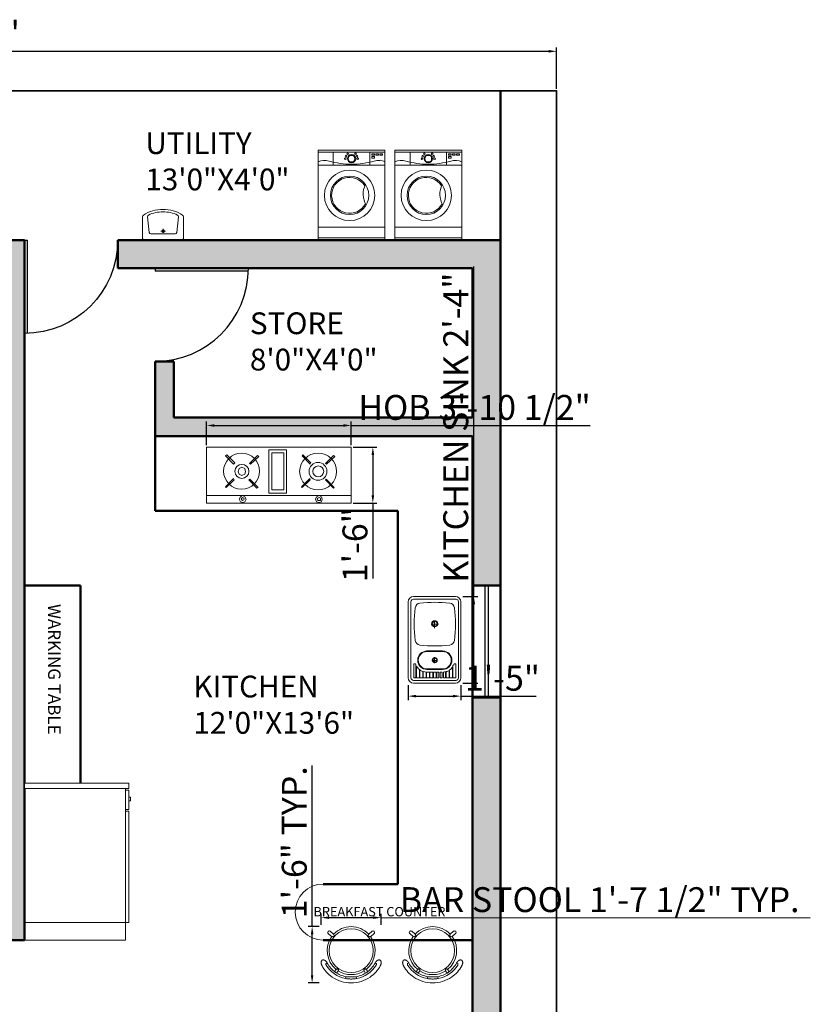
# Model space of a CAD drawing. Units: inches. Extents: x 1986 to 21484, y -1816 to 2016.
# Tile 41 of 85: x 2230 to 2484, y 1607 to 1924. Entities that reach past the tile are written whole.
import ezdxf

# ---------------------------------------------------------------- set-up
doc = ezdxf.new("R2010")
doc.units = ezdxf.units.IN
doc.set_wipeout_variables(frame=1)
for name, color, linetype, lineweight in [('A-ANNO-DIMS', 2, 'Continuous', 18), ('A-ANNO-TEXT', 7, 'Continuous', 18), ('A-AREA-IDEN', 3, 'Continuous', 18), ('A-DOOR', 3, 'Continuous', 25), ('A-FLOR-FIXT', 8, 'Continuous', 18), ('A-FURN', 8, 'Continuous', 18), ('A-GLAZ', 4, 'Continuous', 25), ('A-WALL', 7, 'Continuous', 50), ('A-WALL-PATT', 8, 'Continuous', 13), ('C-PROP', 7, 'Continuous', 35)]:
    doc.layers.add(name, color=color, linetype=linetype, lineweight=lineweight)
doc.styles.get("Standard").update_dxf_attribs({"font": 'arial.ttf'})
doc.dimstyles.new('ISO-25', dxfattribs={"dimtxt": 8, "dimasz": 2.5, "dimexe": 1.25, "dimexo": 0.625, "dimtad": 1, "dimdec": 1, "dimlunit": 3, "dimtxsty": 'Standard', "dimcen": 2.5, "dimadec": 0, "dimazin": 0, "dimtfac": 1, "dimtdec": 1, "dimtmove": 0, "dimatfit": 3, "dimfxl": 1, "dimarcsym": 0})

# ---------------------------------------------------------------- blocks, each defined once
blk = doc.blocks.new('*D1')
at = {"layer": 'A-ANNO-DIMS', "color": 0, "lineweight": -2, "transparency": 16777216}
for p, q in [((2042.31, 1901.38), (2042.31, 1914.65)), ((2402.31, 1901.38), (2402.31, 1914.65)), ((2044.81, 1913.4), (2399.81, 1913.4))]:
    blk.add_line(p, q, dxfattribs=at)
at = {"layer": 'A-ANNO-DIMS', "color": 0, "transparency": 16777216}
for points in [[(2044.81, 1913.82), (2044.81, 1912.99), (2042.31, 1913.4)], [(2399.81, 1913.82), (2399.81, 1912.99), (2402.31, 1913.4)]]:
    blk.add_solid(points, dxfattribs=at)
at = {"layer": 'Defpoints', "color": 0, "transparency": 16777216}
for p in [(2402.31, 1913.4), (2042.31, 1900.75), (2402.31, 1900.75)]:
    blk.add_point(p, dxfattribs=at)
at = {"layer": 'A-ANNO-DIMS', "color": 0, "transparency": 16777216, "insert": (2222.31, 1918.12), "char_height": 8, "attachment_point": 5}
blk.add_mtext("30'", dxfattribs=at)
blk = doc.blocks.new('D2')
for p, q in [((1722.5, 1505.46), (1722.5, 1475.46)), ((1723.5, 1505.46), (1723.5, 1475.46)), ((1722.5, 1475.46), (1723.5, 1475.46))]:
    blk.add_line(p, q)
blk.add_arc((1722.5, 1475.46), 30, 0, 90)
blk = doc.blocks.new('A$C2EBB240D')
for p, q in [((480, 376), (20, 376)), ((0, 356), (0, 87)), ((61, 90), (82, 282)), ((250, 300), (102, 300)), ((250, 300), (398, 300)), ((439, 90), (418, 282)), ((500, 356), (500, 87))]:
    blk.add_line(p, q)
for points in [[(275, 266), (219, 266)], [(247, 238), (247, 289)]]:
    blk.add_lwpolyline(points)
for centre, radius, start, end in [((20, 356), 20, 90, 180), ((480, 356), 20, 0, 90), ((102, 280), 20, 90, 173.6428), ((247, 266), 16.7, 90, 270), ((247, 266), 10, 90, 270), ((247, 266), 16.7, 270, 90), ((247, 266), 10, 270, 90), ((398, 280), 20, 6.3572, 90), ((20, 87), 20, 180, 237.6892), ((250, 450), 450, 237.6892, 270), ((81, 88), 20, 173.6428, 244.9796), ((250, 450), 420, 244.9796, 270), ((250, 450), 450, 270, 302.3108), ((250, 450), 420, 270, 295.0204), ((419, 88), 20, 295.0204, 6.3572), ((480, 87), 20, 302.3108, 0)]:
    blk.add_arc(centre, radius, start, end)
blk = doc.blocks.new('SILLA 01')
for p, q in [((-0.118, 0.2405), (-0.1161, 0.2412)), ((-0.1161, 0.2412), (-0.1143, 0.2419)), ((-0.1143, 0.2419), (-0.1124, 0.2426)), ((-0.1124, 0.2426), (-0.1104, 0.2431)), ((-0.1104, 0.2431), (-0.1085, 0.2437)), ((-0.1085, 0.2437), (-0.1069, 0.244)), ((-0.1069, 0.244), (-0.1053, 0.2444)), ((-0.1053, 0.2444), (-0.1037, 0.2446)), ((-0.1037, 0.2446), (-0.102, 0.2448)), ((-0.102, 0.2448), (-0.1004, 0.2449)), ((-0.1004, 0.2449), (-0.0987, 0.245)), ((-0.0987, 0.245), (-0.0971, 0.245)), ((-0.0971, 0.245), (-0.0954, 0.2449)), ((-0.0954, 0.2449), (-0.0939, 0.2448)), ((-0.0939, 0.2448), (-0.0924, 0.2446)), ((-0.0924, 0.2446), (-0.0908, 0.2443)), ((-0.0908, 0.2443), (-0.0893, 0.2439)), ((-0.0893, 0.2439), (-0.0878, 0.2435)), ((-0.0878, 0.2435), (-0.0864, 0.243)), ((-0.0864, 0.243), (-0.0849, 0.2423)), ((-0.0849, 0.2423), (-0.0836, 0.2417)), ((-0.0836, 0.2417), (-0.0826, 0.2411)), ((-0.2162, 0.1544), (-0.2068, 0.1672)), ((-0.2068, 0.1672), (-0.1968, 0.1793)), ((-0.1968, 0.1793), (-0.186, 0.1909)), ((-0.186, 0.1909), (-0.1746, 0.2017)), ((-0.1746, 0.2017), (-0.1626, 0.2119)), ((-0.1744, 0.1565), (-0.1571, 0.1744)), ((-0.1626, 0.2119), (-0.1501, 0.2213)), ((-0.1571, 0.1744), (-0.1381, 0.1904)), ((-0.1525, 0.1566), (-0.1432, 0.1655)), ((-0.1501, 0.2213), (-0.137, 0.23)), ((-0.1432, 0.1655), (-0.1334, 0.1739)), ((-0.1381, 0.1904), (-0.1176, 0.2043)), ((-0.137, 0.23), (-0.1234, 0.2379)), ((-0.1334, 0.1739), (-0.123, 0.1816)), ((-0.1234, 0.2379), (-0.1216, 0.2388)), ((-0.123, 0.1816), (-0.1123, 0.1887)), ((-0.1216, 0.2388), (-0.1198, 0.2397)), ((-0.1198, 0.2397), (-0.118, 0.2405)), ((-0.1176, 0.2043), (-0.1159, 0.2052)), ((-0.1159, 0.2052), (-0.1142, 0.2058)), ((-0.1142, 0.2058), (-0.1123, 0.2062)), ((-0.1123, 0.2062), (-0.1104, 0.2063)), ((-0.1123, 0.1887), (-0.1012, 0.1952)), ((-0.1104, 0.2063), (-0.1086, 0.2062)), ((-0.1086, 0.2062), (-0.1067, 0.2058)), ((-0.1067, 0.2058), (-0.105, 0.2051)), ((-0.105, 0.2051), (-0.1033, 0.2042)), ((-0.0994, 0.1962), (-0.1012, 0.1952)), ((-0.0977, 0.1972), (-0.0994, 0.1962)), ((-0.096, 0.1983), (-0.0977, 0.1972)), ((-0.0943, 0.1994), (-0.096, 0.1983)), ((-0.0927, 0.2006), (-0.0943, 0.1994)), ((-0.0911, 0.2019), (-0.0927, 0.2006)), ((-0.0896, 0.2031), (-0.0911, 0.2019)), ((-0.0881, 0.2045), (-0.0896, 0.2031)), ((-0.0869, 0.2056), (-0.0881, 0.2045)), ((-0.0857, 0.2068), (-0.0869, 0.2056)), ((-0.0846, 0.208), (-0.0857, 0.2068)), ((-0.0835, 0.2093), (-0.0846, 0.208)), ((-0.0825, 0.2106), (-0.0835, 0.2093)), ((-0.0826, 0.2411), (-0.0817, 0.2405)), ((-0.0815, 0.212), (-0.0825, 0.2106)), ((-0.0817, 0.2405), (-0.0808, 0.2398)), ((-0.0806, 0.2133), (-0.0815, 0.212)), ((-0.0808, 0.2398), (-0.08, 0.239)), ((-0.0797, 0.2148), (-0.0806, 0.2133)), ((-0.08, 0.239), (-0.0792, 0.2382)), ((-0.0789, 0.2161), (-0.0797, 0.2148)), ((-0.0792, 0.2382), (-0.0785, 0.2373)), ((-0.0782, 0.2176), (-0.0789, 0.2161)), ((-0.0785, 0.2373), (-0.0779, 0.2364)), ((-0.0776, 0.219), (-0.0782, 0.2176)), ((-0.0779, 0.2364), (-0.0773, 0.2354)), ((-0.0771, 0.2205), (-0.0776, 0.219)), ((-0.0773, 0.2354), (-0.0769, 0.2344)), ((-0.0766, 0.222), (-0.0771, 0.2205)), ((-0.0769, 0.2344), (-0.0764, 0.2333)), ((-0.0762, 0.2235), (-0.0766, 0.222)), ((-0.0764, 0.2333), (-0.0761, 0.2322)), ((-0.0759, 0.2251), (-0.0762, 0.2235)), ((-0.0761, 0.2322), (-0.0759, 0.2311)), ((-0.0759, 0.2311), (-0.0757, 0.23)), ((-0.0757, 0.2266), (-0.0759, 0.2251)), ((-0.0757, 0.23), (-0.0756, 0.2289)), ((-0.0756, 0.2278), (-0.0757, 0.2266)), ((-0.0756, 0.2289), (-0.0756, 0.2278)), ((0.1165, 0.1601), (0.1387, 0.1871)), ((0.1577, 0.1709), (0.1354, 0.1439)), ((0.1387, 0.1871), (0.1425, 0.1901)), ((0.1425, 0.1901), (0.1471, 0.1915)), ((0.1471, 0.1915), (0.1519, 0.191)), ((0.1519, 0.191), (0.1561, 0.1886)), ((0.1561, 0.1886), (0.1592, 0.1848)), ((0.16, 0.1752), (0.1577, 0.1709)), ((0.1592, 0.1848), (0.1605, 0.1801)), ((0.1605, 0.1801), (0.16, 0.1752)), ((-0.2571, 0.0611), (-0.2518, 0.081)), ((-0.2518, 0.081), (-0.245, 0.1003)), ((-0.245, 0.1003), (-0.2367, 0.1191)), ((-0.2367, 0.1191), (-0.2271, 0.1372)), ((-0.2271, 0.1372), (-0.2162, 0.1544)), ((-0.2221, 0.0696), (-0.2136, 0.0931)), ((-0.2136, 0.0931), (-0.2028, 0.1156)), ((-0.2034, 0.0756), (-0.1993, 0.0864)), ((-0.2028, 0.1156), (-0.1896, 0.1368)), ((-0.1993, 0.0864), (-0.1945, 0.0969)), ((-0.1945, 0.0969), (-0.1893, 0.1071)), ((-0.1896, 0.1368), (-0.1744, 0.1565)), ((-0.1893, 0.1071), (-0.1835, 0.1171)), ((-0.1835, 0.1171), (-0.1773, 0.1267)), ((-0.1828, 0.1184), (-0.1651, 0.1058)), ((-0.1773, 0.1267), (-0.1696, 0.1372)), ((-0.1538, 0.1223), (-0.1714, 0.1348)), ((-0.1696, 0.1372), (-0.1614, 0.1472)), ((-0.1616, 0.1042), (-0.1651, 0.1058)), ((-0.1577, 0.1041), (-0.1616, 0.1042)), ((-0.1614, 0.1472), (-0.1525, 0.1566)), ((-0.1541, 0.1055), (-0.1577, 0.1041)), ((-0.1513, 0.1083), (-0.1541, 0.1055)), ((-0.1538, 0.1223), (-0.1511, 0.1194)), ((-0.1498, 0.1118), (-0.1513, 0.1083)), ((-0.1511, 0.1194), (-0.1497, 0.1158)), ((-0.1497, 0.1158), (-0.1498, 0.1118)), ((0.1136, 0.1509), (0.1141, 0.1558)), ((0.115, 0.1462), (0.1136, 0.1509)), ((0.1141, 0.1558), (0.1165, 0.1601)), ((0.118, 0.1423), (0.115, 0.1462)), ((0.1222, 0.14), (0.118, 0.1423)), ((0.127, 0.1394), (0.1222, 0.14)), ((0.1317, 0.1408), (0.127, 0.1394)), ((0.1354, 0.1439), (0.1317, 0.1408)), ((-0.264, 0), (-0.2632, 0.0205)), ((-0.2632, -0.0205), (-0.264, 0)), ((-0.2632, 0.0205), (-0.2609, 0.041)), ((-0.2609, 0.041), (-0.2571, 0.0611)), ((-0.2318, 0), (-0.2317, 0.0057)), ((-0.2317, -0.0057), (-0.2318, 0)), ((-0.2317, 0.0057), (-0.2315, 0.0114)), ((-0.2315, 0.0114), (-0.2312, 0.017)), ((-0.2312, 0.017), (-0.2307, 0.0227)), ((-0.2307, 0.0227), (-0.2301, 0.0283)), ((-0.2301, 0.0283), (-0.2294, 0.034)), ((-0.2294, 0.034), (-0.2285, 0.0396)), ((-0.2285, 0.0396), (-0.2275, 0.0452)), ((-0.2281, 0.0453), (-0.2221, 0.0696)), ((-0.2125, 0.0422), (-0.2275, 0.0452)), ((-0.2125, 0.0422), (-0.2101, 0.0535)), ((-0.2125, 0.0422), (-0.2125, -0.0422)), ((-0.2101, 0.0535), (-0.207, 0.0646)), ((-0.207, 0.0646), (-0.2034, 0.0756)), ((-0.2609, -0.041), (-0.2632, -0.0205)), ((-0.2571, -0.0611), (-0.2609, -0.041)), ((-0.2518, -0.081), (-0.2571, -0.0611)), ((-0.2315, -0.0114), (-0.2317, -0.0057)), ((-0.2312, -0.017), (-0.2315, -0.0114)), ((-0.2307, -0.0227), (-0.2312, -0.017)), ((-0.2301, -0.0283), (-0.2307, -0.0227)), ((-0.2294, -0.034), (-0.2301, -0.0283)), ((-0.2285, -0.0396), (-0.2294, -0.034)), ((-0.2275, -0.0452), (-0.2285, -0.0396)), ((-0.2221, -0.0696), (-0.2281, -0.0453)), ((-0.2125, -0.0422), (-0.2275, -0.0452)), ((-0.2136, -0.0931), (-0.2221, -0.0696)), ((-0.2101, -0.0535), (-0.2125, -0.0422)), ((-0.207, -0.0646), (-0.2101, -0.0535)), ((-0.2034, -0.0756), (-0.207, -0.0646)), ((-0.1993, -0.0864), (-0.2034, -0.0756)), ((-0.245, -0.1003), (-0.2518, -0.081)), ((-0.2367, -0.1191), (-0.245, -0.1003)), ((-0.2271, -0.1372), (-0.2367, -0.1191)), ((-0.2162, -0.1544), (-0.2271, -0.1372)), ((-0.2068, -0.1672), (-0.2162, -0.1544)), ((-0.2028, -0.1156), (-0.2136, -0.0931)), ((-0.1896, -0.1368), (-0.2028, -0.1156)), ((-0.1945, -0.0969), (-0.1993, -0.0864)), ((-0.1893, -0.1071), (-0.1945, -0.0969)), ((-0.1744, -0.1565), (-0.1896, -0.1368)), ((-0.1835, -0.1171), (-0.1893, -0.1071)), ((-0.1773, -0.1267), (-0.1835, -0.1171)), ((-0.1828, -0.1184), (-0.1651, -0.1058)), ((-0.1696, -0.1372), (-0.1773, -0.1267)), ((-0.1571, -0.1744), (-0.1744, -0.1565)), ((-0.1538, -0.1223), (-0.1714, -0.1348)), ((-0.1614, -0.1472), (-0.1696, -0.1372)), ((-0.1651, -0.1058), (-0.1616, -0.1042)), ((-0.1616, -0.1042), (-0.1577, -0.1041)), ((-0.1525, -0.1566), (-0.1614, -0.1472)), ((-0.1577, -0.1041), (-0.1541, -0.1055)), ((-0.1541, -0.1055), (-0.1513, -0.1083)), ((-0.1511, -0.1194), (-0.1538, -0.1223)), ((-0.1432, -0.1655), (-0.1525, -0.1566)), ((-0.1513, -0.1083), (-0.1498, -0.1118)), ((-0.1497, -0.1158), (-0.1511, -0.1194)), ((-0.1498, -0.1118), (-0.1497, -0.1158)), ((0.1136, -0.1509), (0.115, -0.1462)), ((0.1141, -0.1558), (0.1136, -0.1509)), ((0.1165, -0.1601), (0.1141, -0.1558)), ((0.115, -0.1462), (0.118, -0.1423)), ((0.1165, -0.1601), (0.1387, -0.1871)), ((0.118, -0.1423), (0.1222, -0.14)), ((0.1222, -0.14), (0.127, -0.1394)), ((0.127, -0.1394), (0.1317, -0.1408)), ((0.1317, -0.1408), (0.1354, -0.1439)), ((0.1577, -0.1709), (0.1354, -0.1439)), ((-0.1968, -0.1793), (-0.2068, -0.1672)), ((-0.186, -0.1909), (-0.1968, -0.1793)), ((-0.1746, -0.2017), (-0.186, -0.1909)), ((-0.1626, -0.2119), (-0.1746, -0.2017)), ((-0.1501, -0.2213), (-0.1626, -0.2119)), ((-0.1381, -0.1904), (-0.1571, -0.1744)), ((-0.137, -0.23), (-0.1501, -0.2213)), ((-0.1334, -0.1739), (-0.1432, -0.1655)), ((-0.1176, -0.2043), (-0.1381, -0.1904)), ((-0.1234, -0.2379), (-0.137, -0.23)), ((-0.123, -0.1816), (-0.1334, -0.1739)), ((-0.1216, -0.2388), (-0.1234, -0.2379)), ((-0.1123, -0.1887), (-0.123, -0.1816)), ((-0.1198, -0.2397), (-0.1216, -0.2388)), ((-0.118, -0.2405), (-0.1198, -0.2397)), ((-0.1161, -0.2412), (-0.118, -0.2405)), ((-0.1159, -0.2052), (-0.1176, -0.2043)), ((-0.1142, -0.2058), (-0.1159, -0.2052)), ((-0.1123, -0.2062), (-0.1142, -0.2058)), ((-0.1012, -0.1952), (-0.1123, -0.1887)), ((-0.1104, -0.2063), (-0.1123, -0.2062)), ((-0.1086, -0.2062), (-0.1104, -0.2063)), ((-0.1067, -0.2058), (-0.1086, -0.2062)), ((-0.105, -0.2051), (-0.1067, -0.2058)), ((-0.1033, -0.2042), (-0.105, -0.2051)), ((-0.1012, -0.1952), (-0.0994, -0.1962)), ((-0.0994, -0.1962), (-0.0977, -0.1972)), ((-0.0977, -0.1972), (-0.096, -0.1983)), ((-0.096, -0.1983), (-0.0943, -0.1994)), ((-0.0943, -0.1994), (-0.0927, -0.2006)), ((-0.0927, -0.2006), (-0.0911, -0.2019)), ((-0.0911, -0.2019), (-0.0896, -0.2031)), ((-0.0896, -0.2031), (-0.0881, -0.2045)), ((-0.0881, -0.2045), (-0.0869, -0.2056)), ((-0.0869, -0.2056), (-0.0857, -0.2068)), ((-0.0857, -0.2068), (-0.0846, -0.208)), ((-0.0846, -0.208), (-0.0835, -0.2093)), ((-0.0826, -0.2411), (-0.0836, -0.2417)), ((-0.0835, -0.2093), (-0.0825, -0.2106)), ((-0.0817, -0.2405), (-0.0826, -0.2411)), ((-0.0825, -0.2106), (-0.0815, -0.212)), ((-0.0808, -0.2398), (-0.0817, -0.2405)), ((-0.0815, -0.212), (-0.0806, -0.2133)), ((-0.08, -0.239), (-0.0808, -0.2398)), ((-0.0806, -0.2133), (-0.0797, -0.2148)), ((-0.0792, -0.2382), (-0.08, -0.239)), ((-0.0797, -0.2148), (-0.0789, -0.2161)), ((-0.0785, -0.2373), (-0.0792, -0.2382)), ((-0.0789, -0.2161), (-0.0782, -0.2176)), ((-0.0779, -0.2364), (-0.0785, -0.2373)), ((-0.0782, -0.2176), (-0.0776, -0.219)), ((-0.0773, -0.2354), (-0.0779, -0.2364)), ((-0.0776, -0.219), (-0.0771, -0.2205)), ((-0.0769, -0.2344), (-0.0773, -0.2354)), ((-0.0771, -0.2205), (-0.0766, -0.222)), ((-0.0764, -0.2333), (-0.0769, -0.2344)), ((-0.0766, -0.222), (-0.0762, -0.2235)), ((-0.0761, -0.2322), (-0.0764, -0.2333)), ((-0.0762, -0.2235), (-0.0759, -0.2251)), ((-0.0759, -0.2311), (-0.0761, -0.2322)), ((-0.0759, -0.2251), (-0.0757, -0.2266)), ((-0.0757, -0.23), (-0.0759, -0.2311)), ((-0.0757, -0.2266), (-0.0756, -0.2278)), ((-0.0756, -0.2289), (-0.0757, -0.23)), ((-0.0756, -0.2278), (-0.0756, -0.2289)), ((0.1425, -0.1901), (0.1387, -0.1871)), ((0.1471, -0.1915), (0.1425, -0.1901)), ((0.1519, -0.191), (0.1471, -0.1915)), ((0.1561, -0.1886), (0.1519, -0.191)), ((0.1592, -0.1848), (0.1561, -0.1886)), ((0.1577, -0.1709), (0.16, -0.1752)), ((0.1605, -0.1801), (0.1592, -0.1848)), ((0.16, -0.1752), (0.1605, -0.1801)), ((-0.1143, -0.2419), (-0.1161, -0.2412)), ((-0.1124, -0.2426), (-0.1143, -0.2419)), ((-0.1104, -0.2431), (-0.1124, -0.2426)), ((-0.1085, -0.2437), (-0.1104, -0.2431)), ((-0.1069, -0.244), (-0.1085, -0.2437)), ((-0.1053, -0.2444), (-0.1069, -0.244)), ((-0.1037, -0.2446), (-0.1053, -0.2444)), ((-0.102, -0.2448), (-0.1037, -0.2446)), ((-0.1004, -0.2449), (-0.102, -0.2448)), ((-0.0987, -0.245), (-0.1004, -0.2449)), ((-0.0971, -0.245), (-0.0987, -0.245)), ((-0.0954, -0.2449), (-0.0971, -0.245)), ((-0.0939, -0.2448), (-0.0954, -0.2449)), ((-0.0924, -0.2446), (-0.0939, -0.2448)), ((-0.0908, -0.2443), (-0.0924, -0.2446)), ((-0.0893, -0.2439), (-0.0908, -0.2443)), ((-0.0878, -0.2435), (-0.0893, -0.2439)), ((-0.0864, -0.243), (-0.0878, -0.2435)), ((-0.0849, -0.2423), (-0.0864, -0.243)), ((-0.0836, -0.2417), (-0.0849, -0.2423))]:
    blk.add_line(p, q)
blk.add_circle((0, 0), 0.1793)
for start, end in [(53.88178, 141.5278), (147.34891, 212.65109), (313.19891, 46.80109), (218.4722, 306.11822)]:
    blk.add_arc((0, 0), 0.196, start, end)
blk = doc.blocks.new('gas 1')
for points in [[(35.93, -1.87), (35.93, 0), (0, 0), (0, -1.87)], [(8.12, -0.94), (8.44, -1.56), (8.91, -1.87), (9.53, -1.56), (9.84, -0.94), (9.53, -0.31), (8.91, -0.16), (8.44, -0.31)], [(8.59, -0.94), (8.75, -1.25), (8.91, -1.41), (9.22, -1.25), (9.37, -0.94), (9.22, -0.78), (8.91, -0.62), (8.75, -0.78)], [(27.03, -0.94), (27.34, -1.56), (27.97, -1.87), (28.59, -1.56), (28.75, -0.94), (28.59, -0.31), (27.97, -0.16), (27.34, -0.31)], [(27.5, -0.94), (27.65, -1.25), (27.97, -1.41), (28.28, -1.25), (28.28, -0.94), (28.28, -0.62), (27.97, -0.62), (27.65, -0.62)], [(4.84, -3.91), (4.69, -4.06), (6.72, -6.09), (6.87, -5.78)], [(12.81, -3.91), (12.5, -3.75), (10.47, -5.78), (10.78, -5.94)], [(19.84, -13.28), (15.47, -13.28), (15.47, -2.5), (19.84, -2.5)], [(19.22, -12.5), (16.25, -12.5), (16.25, -3.28), (19.22, -3.28)], [(23.75, -3.91), (23.59, -4.06), (25.62, -6.09), (25.78, -5.78)], [(31.71, -3.91), (31.56, -3.75), (29.53, -5.78), (29.68, -5.94)], [(7.81, -7.81), (8.12, -8.59), (8.75, -8.91), (9.53, -8.59), (9.69, -7.81), (9.53, -7.19), (8.75, -6.87), (8.12, -7.19)], [(7.03, -10), (6.72, -9.69), (4.69, -11.72), (5, -12.03)], [(12.97, -11.56), (10.94, -9.69), (10.62, -9.84), (12.65, -11.87)], [(23.75, -11.72), (23.9, -12.03), (25.93, -10), (25.78, -9.69)], [(31.87, -11.56), (29.84, -9.69), (29.53, -9.84), (31.56, -11.87)]]:
    blk.add_lwpolyline(points, close=True)
blk.add_lwpolyline([(35.93, -1.87), (35.93, -13.9), (0, -13.9), (0, -1.87)])
for centre, radius in [((8.7, -7.92), 4.48), ((27.7, -7.86), 4.58), ((8.77, -7.89), 1.74), ((27.69, -7.89), 2.22), ((27.76, -7.89), 1.35)]:
    blk.add_circle(centre, radius)
blk = doc.blocks.new('sink 1')
for points in [[(-7.34, 1.48), (-7.34, 22.73)], [(-6.56, 1.48), (-6.56, 22.73)], [(5.86, 24.22), (-5.86, 24.22)], [(6.01, 23.43), (-5.86, 23.43)], [(6.72, 1.48), (6.72, 22.73)], [(7.34, 1.48), (7.34, 22.73)], [(0, 15.39), (0, 17.42)], [(1.09, 16.48), (-0.94, 16.48)], [(-2.09, 8.99), (2.28, 8.99)], [(-2.09, 8.84), (2.28, 8.84)], [(0.78, 6.33), (-0.78, 6.33)], [(0, 5.55), (0, 7.26)], [(-5.78, 5.39), (-5.78, 5.39)], [(-5.31, 5.39), (-5.31, 5.39)], [(-5.16, 4.92), (-5.16, 4.92)], [(-5, 1.48), (-5, 4.69)], [(-5, 1.48), (-4.22, 1.48), (-4.22, 3.83)], [(-4.84, 4.45), (-4.84, 4.45)], [(-4.22, 3.83), (-4.22, 3.83)], [(-4.06, 1.48), (-4.06, 3.69)], [(-4.06, 1.48), (-3.28, 1.48), (-3.28, 3.27)], [(-3.91, 3.52), (-3.91, 3.52)], [(-3.28, 3.2), (-3.28, 3.2)], [(-3.12, 3.2), (-3.12, 3.2)], [(-2.34, 3.05), (-2.34, 3.05)], [(-2.19, 3.05), (-2.19, 3.05)], [(-2.09, 3.99), (2.28, 3.99)], [(-2.09, 3.84), (2.28, 3.84)], [(-1.41, 3.05), (-1.41, 3.05)], [(-1.25, 3.05), (-1.25, 3.05)], [(-0.47, 1.48), (-1.25, 1.48), (-1.25, 3.05), (-0.47, 3.05)], [(-0.62, 3.05), (-0.62, 3.05)], [(-0.47, 1.48), (-0.47, 3.05)], [(-0.31, 3.05), (-0.31, 3.05)], [(0.47, 1.48), (-0.31, 1.48), (-0.31, 3.05), (0.47, 3.05)], [(0.31, 3.05), (0.31, 3.05)], [(0.47, 1.48), (0.47, 3.05)], [(0.62, 3.05), (0.62, 3.05)], [(1.25, 3.05), (1.25, 3.05)], [(1.56, 3.05), (1.56, 3.05)], [(2.19, 3.05), (2.19, 3.05)], [(2.5, 3.05), (2.5, 3.05)], [(3.12, 3.2), (3.12, 3.2)], [(3.28, 1.48), (4.06, 1.48), (4.06, 3.57)], [(3.28, 1.48), (3.28, 3.2)], [(3.44, 3.2), (3.44, 3.2)], [(4.06, 3.52), (4.06, 3.52)], [(4.22, 1.48), (4.22, 3.67)], [(4.37, 3.83), (4.37, 3.83)], [(5, 4.45), (5, 4.45)], [(5.16, 4.92), (5.16, 4.92)], [(5.94, 5.39), (5.94, 5.39)], [(6.01, 0.78), (-5.86, 0.78)], [(5.86, 0), (-5.86, 0)], [(-5.78, 1.48), (-5.78, 1.48)], [(-5.16, 1.48), (-5.16, 1.48)], [(-4.84, 1.48), (-4.84, 1.48)], [(-4.22, 1.48), (-4.22, 1.48)], [(-3.91, 1.48), (-3.91, 1.48)], [(-3.28, 1.48), (-3.28, 1.48)], [(-3.12, 1.48), (-3.12, 1.48)], [(-2.34, 1.48), (-2.34, 1.48)], [(-2.19, 1.48), (-2.19, 1.48)], [(-1.41, 1.48), (-1.41, 1.48)], [(-1.25, 1.48), (-1.25, 1.48)], [(-0.62, 1.48), (-0.62, 1.48)], [(-0.31, 1.48), (-0.31, 1.48)], [(0.31, 1.48), (0.31, 1.48)], [(0.62, 1.48), (0.62, 1.48)], [(1.25, 1.48), (1.25, 1.48)], [(1.56, 1.48), (1.56, 1.48)], [(2.19, 1.48), (2.19, 1.48)], [(2.5, 1.48), (2.5, 1.48)], [(3.12, 1.48), (3.12, 1.48)], [(3.44, 1.48), (3.44, 1.48)], [(4.06, 1.48), (4.06, 1.48)], [(4.37, 1.48), (4.37, 1.48)], [(5, 1.48), (5, 1.48)], [(5.16, 1.48), (5.16, 1.48)], [(5.94, 1.48), (5.94, 1.48)]]:
    blk.add_lwpolyline(points)
for points in [[(-5.16, 4.92), (-5.16, 1.48), (-5.78, 1.48), (-5.78, 5.39), (-5.31, 5.39, -0.068511), (-5.16, 4.92)], [(4.06, 3.57, -0.061679), (3.32, 3.22)], [(4.22, 1.48), (5, 1.48), (5, 4.45, -0.083542), (4.22, 3.67, -0.083542)], [(5.16, 4.92, 0.248301), (5.47, 5.39), (5.94, 5.39), (5.94, 1.48), (5.16, 1.48), (5.16, 4.92)]]:
    blk.add_lwpolyline(points, format="xyb")
for points in [[(-3.12, 3.22), (-3.12, 1.48), (-2.34, 1.48), (-2.34, 3.05, -0.06228)], [(2.5, 3.05), (2.5, 1.48), (3.12, 1.48), (3.12, 3.2, -0.050256)]]:
    blk.add_lwpolyline(points, format="xyb", close=True)
for points in [[(-2.19, 3.05), (-1.41, 3.05), (-1.41, 1.48), (-2.19, 1.48)], [(0.62, 3.05), (1.25, 3.05), (1.25, 1.48), (0.62, 1.48)], [(2.19, 1.48), (2.19, 3.05), (1.56, 3.05), (1.56, 1.48)]]:
    blk.add_lwpolyline(points, close=True)
for centre, radius in [((0.09, 16.57), 0.859), ((0.09, 16.57), 0.703), ((0.09, 6.41), 0.703), ((0.09, 6.41), 0.547)]:
    blk.add_circle(centre, radius)
for centre, radius, start, end in [((-5.86, 22.73), 1.48, 90, 180), ((-5.86, 22.73), 0.703, 90, 180), ((-3.87, 20.82), 1.53, 97.3256, 171.1849), ((0.09, -12.65), 35.23, 83.2159, 96.7841), ((4.06, 20.82), 1.53, 8.8151, 82.6744), ((5.86, 22.73), 1.48, 360, 90), ((6.01, 22.73), 0.703, 0, 90), ((30.19, 16.56), 35.85, 172.7947, 187.4213), ((-30, 16.56), 35.85, 352.5787, 7.2053), ((-3.89, 12.12), 1.48, 187.4212, 263.2159), ((4.08, 12.12), 1.48, 276.7841, 352.5788), ((-2.1, 6.41), 2.58, 90, 270), ((-2.1, 6.41), 2.42, 90, 270), ((0.09, 45.63), 35.23, 263.2159, 276.7841), ((2.28, 6.41), 2.58, 270, 90), ((2.28, 6.41), 2.42, 270, 90), ((-2.15, 6.48), 3.36, 212.1095, 232.0862), ((-2.1, 6.41), 3.36, 234.156, 249.3275), ((2.14, 6.36), 3.36, 289.8633, 290.5971), ((-5.86, 1.48), 1.48, 180, 270), ((-5.86, 1.48), 0.703, 180, 270), ((5.86, 1.48), 1.48, 270, 0), ((6.01, 1.48), 0.703, 270, 360)]:
    blk.add_arc(centre, radius, start, end)
blk = doc.blocks.new('WIN-36')
for p, q in [((0, 36), (0, 0)), ((0, 36), (0, 0)), ((1, 36), (1, 0))]:
    blk.add_line(p, q)
blk = doc.blocks.new('*D113')
at = {"layer": 'A-ANNO-DIMS', "color": 0, "lineweight": -2, "transparency": 16777216}
for p, q in [((2326.66, 1632.69), (2326.67, 1636.21)), ((2345.96, 1632.69), (2345.96, 1636.21)), ((2329.17, 1634.96), (2343.46, 1634.96)), ((2345.96, 1634.96), (2483.83, 1634.92))]:
    blk.add_line(p, q, dxfattribs=at)
at = {"layer": 'A-ANNO-DIMS', "color": 0, "transparency": 16777216}
for points in [[(2329.17, 1635.38), (2329.17, 1634.54), (2326.67, 1634.96)], [(2343.46, 1635.37), (2343.46, 1634.54), (2345.96, 1634.96)]]:
    blk.add_solid(points, dxfattribs=at)
at = {"layer": 'Defpoints', "color": 0, "transparency": 16777216}
for p in [(2345.96, 1634.96), (2326.66, 1632.07), (2345.96, 1632.06)]:
    blk.add_point(p, dxfattribs=at)
at = {"layer": 'A-ANNO-DIMS', "color": 0, "transparency": 16777216, "insert": (2416.15, 1639.7), "char_height": 8, "attachment_point": 5, "rotation": 359.9851}
blk.add_mtext('BAR STOOL 1\'-7 1/2" TYP.', dxfattribs=at)
blk = doc.blocks.new('*D114')
at = {"layer": 'A-ANNO-DIMS', "color": 0, "lineweight": -2, "transparency": 16777216}
for p, q in [((2323.77, 1632.07), (2323.78, 1683.83)), ((2326.04, 1632.07), (2322.52, 1632.07)), ((2323.77, 1616.45), (2323.77, 1629.57)), ((2326.04, 1613.95), (2322.52, 1613.96))]:
    blk.add_line(p, q, dxfattribs=at)
at = {"layer": 'A-ANNO-DIMS', "color": 0, "transparency": 16777216}
for points in [[(2323.35, 1629.57), (2324.19, 1629.57), (2323.77, 1632.07)], [(2323.35, 1616.45), (2324.18, 1616.45), (2323.77, 1613.95)]]:
    blk.add_solid(points, dxfattribs=at)
at = {"layer": 'Defpoints', "color": 0, "transparency": 16777216}
for p in [(2323.77, 1632.07), (2326.66, 1632.07), (2326.66, 1613.95)]:
    blk.add_point(p, dxfattribs=at)
at = {"layer": 'A-ANNO-DIMS', "color": 0, "transparency": 16777216, "insert": (2319.07, 1659.2), "char_height": 8, "attachment_point": 5, "rotation": 89.9851}
blk.add_mtext('1\'-6" TYP.', dxfattribs=at)
blk = doc.blocks.new('*D121')
at = {"layer": 'A-ANNO-DIMS', "color": 0, "lineweight": -2, "transparency": 16777216}
for p, q in [((2289.87, 1786.8), (2289.87, 1794.39)), ((2336.31, 1786.8), (2336.31, 1794.39)), ((2292.37, 1793.14), (2333.81, 1793.14)), ((2336.31, 1793.14), (2413.08, 1793.14))]:
    blk.add_line(p, q, dxfattribs=at)
at = {"layer": 'A-ANNO-DIMS', "color": 0, "transparency": 16777216}
for points in [[(2292.37, 1793.56), (2292.37, 1792.72), (2289.87, 1793.14)], [(2333.81, 1793.56), (2333.81, 1792.72), (2336.31, 1793.14)]]:
    blk.add_solid(points, dxfattribs=at)
at = {"layer": 'Defpoints', "color": 0, "transparency": 16777216}
for p in [(2336.31, 1793.14), (2289.87, 1786.17), (2336.31, 1786.17)]:
    blk.add_point(p, dxfattribs=at)
at = {"layer": 'A-ANNO-DIMS', "color": 0, "transparency": 16777216, "insert": (2375.95, 1797.91), "char_height": 8, "attachment_point": 5}
blk.add_mtext('HOB 3\'-10 1/2"', dxfattribs=at)
blk = doc.blocks.new('*D122')
at = {"layer": 'A-ANNO-DIMS', "color": 0, "lineweight": -2, "transparency": 16777216}
for p, q in [((2336.94, 1786.17), (2344.53, 1786.17)), ((2343.28, 1783.67), (2343.28, 1770.7)), ((2336.94, 1768.2), (2344.53, 1768.2)), ((2343.28, 1768.2), (2343.28, 1743.94))]:
    blk.add_line(p, q, dxfattribs=at)
at = {"layer": 'A-ANNO-DIMS', "color": 0, "transparency": 16777216}
for points in [[(2342.86, 1783.67), (2343.7, 1783.67), (2343.28, 1786.17)], [(2342.86, 1770.7), (2343.7, 1770.7), (2343.28, 1768.2)]]:
    blk.add_solid(points, dxfattribs=at)
at = {"layer": 'Defpoints', "color": 0, "transparency": 16777216}
for p in [(2336.31, 1786.17), (2336.31, 1768.2), (2343.28, 1768.2)]:
    blk.add_point(p, dxfattribs=at)
at = {"layer": 'A-ANNO-DIMS', "color": 0, "transparency": 16777216, "insert": (2338.57, 1754.82), "char_height": 8, "attachment_point": 5, "rotation": 90}
blk.add_mtext('1\'-6"', dxfattribs=at)
blk = doc.blocks.new('*D123')
at = {"layer": 'A-ANNO-DIMS', "color": 0, "lineweight": -2, "transparency": 16777216}
for p, q in [((2375.71, 1738.2), (2375.71, 1844.21)), ((2372.15, 1738.2), (2376.96, 1738.2)), ((2375.71, 1712.83), (2375.71, 1735.7)), ((2372.15, 1710.33), (2376.96, 1710.33))]:
    blk.add_line(p, q, dxfattribs=at)
at = {"layer": 'A-ANNO-DIMS', "color": 0, "transparency": 16777216}
for points in [[(2375.29, 1735.7), (2376.12, 1735.7), (2375.71, 1738.2)], [(2375.29, 1712.83), (2376.12, 1712.83), (2375.71, 1710.33)]]:
    blk.add_solid(points, dxfattribs=at)
at = {"layer": 'Defpoints', "color": 0, "transparency": 16777216}
for p in [(2371.53, 1738.2), (2375.71, 1738.2), (2371.53, 1710.33)]:
    blk.add_point(p, dxfattribs=at)
at = {"layer": 'A-ANNO-DIMS', "color": 0, "transparency": 16777216, "insert": (2370.95, 1792.45), "char_height": 8, "attachment_point": 5, "rotation": 90}
blk.add_mtext('KITCHEN SINK 2\'-4"', dxfattribs=at)
blk = doc.blocks.new('*D124')
at = {"layer": 'A-ANNO-DIMS', "color": 0, "lineweight": -2, "transparency": 16777216}
for p, q in [((2354.63, 1709.71), (2354.63, 1704.9)), ((2371.53, 1709.71), (2371.53, 1704.9)), ((2357.13, 1706.15), (2369.03, 1706.15)), ((2371.53, 1706.15), (2395.79, 1706.15))]:
    blk.add_line(p, q, dxfattribs=at)
at = {"layer": 'A-ANNO-DIMS', "color": 0, "transparency": 16777216}
for points in [[(2357.13, 1706.57), (2357.13, 1705.73), (2354.63, 1706.15)], [(2369.03, 1706.57), (2369.03, 1705.73), (2371.53, 1706.15)]]:
    blk.add_solid(points, dxfattribs=at)
at = {"layer": 'Defpoints', "color": 0, "transparency": 16777216}
for p in [(2354.63, 1710.33), (2371.53, 1710.33), (2371.53, 1706.15)]:
    blk.add_point(p, dxfattribs=at)
at = {"layer": 'A-ANNO-DIMS', "color": 0, "transparency": 16777216, "insert": (2384.91, 1710.86), "char_height": 8, "attachment_point": 5}
blk.add_mtext('1\'-5"', dxfattribs=at)

msp = doc.modelspace()

# ---------------------------------------------------------------- hatches: boundary and pattern name
at = {"layer": 'A-WALL-PATT'}
h = msp.add_hatch(color=256, dxfattribs=at)
h.dxf.hatch_style = 1
h.paths.add_polyline_path([(2087.31, 1843.75), (2135.31, 1843.75), (2135.31, 1852.75), (2078.31, 1852.75), (2078.31, 1753.75), (2087.31, 1753.75)])
h.paths.add_polyline_path([(2231.31, 1852.75), (2177.31, 1852.75), (2177.31, 1843.75), (2225.31, 1843.75), (2225.31, 1627.75), (2231.31, 1627.75), (2231.31, 1633.35), (2231.31, 1676.45), (2231.31, 1678.13)])
h.paths.add_polyline_path([(2384.31, 1852.75), (2261.31, 1852.75), (2261.31, 1843.75), (2375.31, 1843.75), (2375.31, 1795.75), (2279.31, 1795.75), (2279.31, 1813.75), (2273.31, 1813.75), (2273.31, 1789.75), (2375.31, 1789.75), (2375.31, 1741.75), (2384.31, 1741.75)])
h.paths.add_polyline_path([(2384.31, 1705.75), (2375.31, 1705.75), (2375.31, 1600.75), (2384.31, 1600.75)])
h.paths.add_polyline_path([(2384.31, 1564.75), (2375.31, 1564.75), (2375.31, 1537.75), (2293.31, 1537.75), (2293.31, 1531.75), (2375.31, 1531.75), (2384.31, 1531.75)])
h.paths.add_polyline_path([(2087.31, 1711.75), (2078.31, 1711.75), (2078.31, 1669.75), (2087.31, 1669.75), (2087.31, 1681.75), (2177.31, 1681.75), (2177.31, 1663.75), (2183.31, 1663.75), (2183.31, 1681.75), (2189.31, 1681.75), (2189.31, 1687.75), (2087.31, 1687.75)])
h.paths.add_polyline_path([(2087.31, 1627.75), (2183.31, 1627.75), (2183.31, 1633.75), (2153.31, 1633.75), (2087.31, 1633.75), (2087.31, 1645.75), (2078.31, 1645.75), (2078.31, 1441.75), (2087.31, 1441.75)])
h.paths.add_polyline_path([(2087.31, 1399.75), (2078.31, 1399.75), (2078.31, 1276.75), (2087.31, 1276.75)])
h.paths.add_polyline_path([(2151.81, 1387.75), (2135.31, 1387.75), (2135.31, 1378.75), (2151.81, 1378.75)])
h.paths.add_polyline_path([(2219.31, 1387.75), (2193.81, 1387.75), (2193.81, 1378.75), (2210.31, 1378.75), (2210.31, 1189.75), (2219.31, 1189.75)])
h.paths.add_polyline_path([(2384.31, 1387.75), (2375.31, 1387.75), (2255.31, 1387.75), (2255.31, 1381.75), (2375.31, 1381.75), (2375.31, 1363.75), (2384.31, 1363.75)])
h.paths.add_polyline_path([(2384.31, 1339.75), (2375.31, 1339.75), (2375.31, 1321.75), (2279.31, 1321.75), (2279.31, 1351.75), (2273.31, 1351.75), (2273.31, 1315.75), (2375.31, 1315.75), (2375.31, 1303.75), (2384.31, 1303.75)])
h.paths.add_polyline_path([(2225.31, 1123.75), (2219.31, 1123.75), (2219.31, 1147.75), (2210.31, 1147.75), (2210.31, 1114.75), (2225.31, 1114.75)])
h.paths.add_polyline_path([(2384.31, 1147.75), (2375.31, 1147.75), (2375.31, 1123.75), (2267.31, 1123.75), (2267.31, 1114.75), (2384.31, 1114.75)])
h.paths.add_polyline_path([(2384.31, 1261.75), (2375.31, 1261.75), (2375.31, 1189.75), (2384.31, 1189.75)])
h.paths.add_polyline_path([(2384.31, 1441.75), (2375.31, 1441.75), (2375.31, 1423.75), (2384.31, 1423.75)])
h.paths.add_polyline_path([(2384.31, 1495.75), (2375.31, 1495.75), (2375.31, 1477.75), (2384.31, 1477.75)])

# ---------------------------------------------------------------- linework, layer by layer
at = {"layer": 'A-FLOR-FIXT'}
for p, q in [((2325.73, 1852.75), (2325.73, 1881.65)), ((2325.73, 1881.65), (2347.18, 1881.65)), ((2325.73, 1880.95), (2347.18, 1880.95)), ((2330.57, 1876.8), (2330.57, 1880.95)), ((2342.34, 1876.8), (2342.34, 1880.95)), ((2347.18, 1852.75), (2347.18, 1881.65)), ((2350.37, 1852.75), (2350.37, 1881.65)), ((2350.37, 1881.65), (2371.83, 1881.65)), ((2350.37, 1880.95), (2371.83, 1880.95)), ((2355.22, 1876.8), (2355.22, 1880.95)), ((2366.98, 1876.8), (2366.98, 1880.95)), ((2371.83, 1852.75), (2371.83, 1881.65)), ((2325.73, 1876.8), (2347.18, 1876.8)), ((2350.37, 1876.8), (2371.83, 1876.8)), ((2325.73, 1856.9), (2347.18, 1856.9)), ((2350.37, 1856.9), (2371.83, 1856.9)), ((2325.73, 1853.44), (2347.18, 1853.44)), ((2325.73, 1852.75), (2347.18, 1852.75)), ((2350.37, 1853.44), (2371.83, 1853.44)), ((2350.37, 1852.75), (2371.83, 1852.75)), ((2231.31, 1676.45), (2231.31, 1678.13)), ((2231.31, 1675.89), (2231.31, 1676.45)), ((2231.31, 1669.73), (2231.31, 1675.89)), ((2231.31, 1669.17), (2231.31, 1669.73)), ((2231.31, 1633.35), (2231.31, 1669.17)), ((2231.31, 1627.75), (2231.31, 1633.35)), ((2231.31, 1627.75), (2263.78, 1627.75))]:
    msp.add_line(p, q, dxfattribs=at)
for points in [[(2342.9, 1880.49), (2343.8, 1880.49), (2343.8, 1879.99), (2342.9, 1879.99)], [(2344.21, 1880.49), (2345.11, 1880.49), (2345.11, 1879.99), (2344.21, 1879.99)], [(2345.53, 1880.49), (2346.43, 1880.49), (2346.43, 1879.99), (2345.53, 1879.99)], [(2367.54, 1880.49), (2368.44, 1880.49), (2368.44, 1879.99), (2367.54, 1879.99)], [(2368.86, 1880.49), (2369.76, 1880.49), (2369.76, 1879.99), (2368.86, 1879.99)], [(2370.18, 1880.49), (2371.08, 1880.49), (2371.08, 1879.99), (2370.18, 1879.99)], [(2342.9, 1879.61), (2343.8, 1879.61), (2343.8, 1879.11), (2342.9, 1879.11)], [(2367.54, 1879.61), (2368.44, 1879.61), (2368.44, 1879.11), (2367.54, 1879.11)]]:
    msp.add_lwpolyline(points, close=True, dxfattribs=at)
for centre, radius in [((2334.66, 1879.69), 0.271), ((2335.18, 1880.43), 0.271), ((2336.45, 1878.9), 1.34), ((2336.45, 1878.9), 1.07), ((2337.71, 1880.43), 0.271), ((2338.19, 1879.69), 0.271), ((2359.3, 1879.69), 0.271), ((2359.83, 1880.43), 0.271), ((2361.1, 1878.9), 1.34), ((2361.1, 1878.9), 1.07), ((2362.36, 1880.43), 0.271), ((2362.84, 1879.69), 0.271), ((2334.41, 1878.9), 0.271), ((2338.44, 1878.9), 0.271), ((2359.05, 1878.9), 0.271), ((2363.09, 1878.9), 0.271), ((2335.81, 1867.11), 8.1), ((2360.45, 1867.11), 8.1), ((2335.81, 1867.11), 6.17), ((2360.45, 1867.11), 6.17)]:
    msp.add_circle(centre, radius, dxfattribs=at)
for centre, radius, start, end in [((2327.8, 1873.44), 4.89, 73.3932, 115.105), ((2336.99, 1907.01), 29.92, 254.9063, 268.9794), ((2335.92, 1907.01), 29.92, 271.0206, 285.0937), ((2345.11, 1873.44), 4.89, 64.895, 106.6068), ((2352.45, 1873.44), 4.89, 73.3932, 115.105), ((2361.63, 1907.01), 29.92, 254.9063, 268.9794), ((2360.57, 1907.01), 29.92, 271.0206, 285.0937), ((2369.75, 1873.44), 4.89, 64.895, 106.6068), ((2335.81, 1867.11), 5.77, 31.8067, 332.1506), ((2347, 1867.5), 6.83, 153.19, 210.7673), ((2360.45, 1867.11), 5.77, 31.8067, 332.1506), ((2371.65, 1867.5), 6.83, 153.19, 210.7673)]:
    msp.add_arc(centre, radius, start, end, dxfattribs=at)
at = {"layer": 'A-FURN'}
msp.add_arc((2327.31, 1636.75), 9, 90, 270, dxfattribs=at)
at = {"layer": 'A-WALL'}
for p, q in [((2384.31, 1900.75), (2384.31, 1114.75)), ((2078.31, 1852.75), (2231.31, 1852.75)), ((2231.31, 1627.75), (2231.31, 1852.75)), ((2261.31, 1843.75), (2261.31, 1852.75)), ((2261.31, 1852.75), (2384.31, 1852.75)), ((2261.31, 1843.75), (2375.31, 1843.75)), ((2375.31, 1843.75), (2375.31, 1795.75)), ((2273.31, 1813.75), (2273.31, 1765.75)), ((2273.31, 1813.75), (2279.31, 1813.75)), ((2279.31, 1813.75), (2279.31, 1795.75)), ((2279.31, 1795.75), (2375.31, 1795.75)), ((2273.31, 1789.75), (2375.31, 1789.75)), ((2375.31, 1789.75), (2375.31, 1537.75)), ((2273.31, 1765.75), (2351.31, 1765.75)), ((2351.31, 1765.75), (2351.31, 1645.75)), ((2231.31, 1741.75), (2249.31, 1741.75)), ((2375.31, 1741.75), (2384.31, 1741.75)), ((2375.31, 1705.75), (2384.31, 1705.75)), ((2327.31, 1645.75), (2351.31, 1645.75)), ((2225.31, 1627.75), (2231.31, 1627.75)), ((2327.31, 1627.75), (2375.31, 1627.75))]:
    msp.add_line(p, q, dxfattribs=at)
at = {"layer": 'C-PROP'}
msp.add_lwpolyline([(2042.31, 1900.75), (2402.31, 1900.75), (2402.31, 1066.75), (2042.31, 1066.75)], close=True, dxfattribs=at)

# ---------------------------------------------------------------- block references
at = {"layer": 'A-DOOR', "xscale": -1, "rotation": 180}
msp.add_blockref('D2', (508.81, 3328.21), dxfattribs=at)
at = {"layer": 'A-DOOR', "rotation": 270}
msp.add_blockref('D2', (797.86, 3566.25), dxfattribs=at)
at = {"layer": 'A-FLOR-FIXT', "rotation": 180}
for name, p, xscale, yscale, zscale in [('A$C2EBB240D', (2282.41, 1862.6), 0.026211548048557, 0.026211548048557, 0.026211548048557), ('gas 1', (2289.87, 1768.2), -1.292580420916565, 1.292580420916565, 1.292580420916565)]:
    msp.add_blockref(name, p, dxfattribs=dict(at, xscale=xscale, yscale=yscale, zscale=zscale))
at = {"layer": 'A-FLOR-FIXT', "xscale": 1.150769176553845, "yscale": 1.150769176553845, "zscale": 1.150769176553845}
msp.add_blockref('sink 1', (2363.08, 1710.33), dxfattribs=at)
at = {"layer": 'A-FURN', "xscale": -39.375, "yscale": 39.375, "zscale": 39.375, "rotation": 269.9851020010651}
for p in [(2336.31, 1624.35), (2362.5, 1624.35)]:
    msp.add_blockref('SILLA 01', p, dxfattribs=at)
at = {"layer": 'A-GLAZ'}
msp.add_blockref('WIN-36', (2379.31, 1705.75), dxfattribs=at)

# ---------------------------------------------------------------- texts
at = {"layer": 'A-ANNO-TEXT', "insert": (2242.94, 1735.75), "char_height": 4, "attachment_point": 1, "rotation": 270}
msp.add_mtext_dynamic_manual_height_columns('{\\fTimes New Roman|b0|i0|c0|p18;WARKING TABLE}', width=105.6127, gutter_width=12.5, heights=[0], dxfattribs=at)
at = {"layer": 'A-ANNO-TEXT', "insert": (2324.21, 1638.37), "char_height": 3, "attachment_point": 1}
msp.add_mtext_dynamic_manual_height_columns('{\\fTimes New Roman|b0|i0|c0|p18;BREAKFAST COUNTER}', width=105.6127, gutter_width=12.5, heights=[0], dxfattribs=at)
at = {"layer": 'A-AREA-IDEN', "char_height": 7, "attachment_point": 1}
for s, insert in [('{\\fTimes New Roman|b0|i0|c0|p18;UTILITY\\P13\'0"X4\'0"}', (2270.17, 1887.39)), ('{\\fTimes New Roman|b0|i0|c0|p18;STORE\\P8\'0"X4\'0"}', (2303.77, 1829.49)), ('{\\fTimes New Roman|b0|i0|c0|p18;KITCHEN\\P12\'0"X13\'6"}', (2285.61, 1712.73))]:
    msp.add_mtext_dynamic_manual_height_columns(s, width=105.6127, gutter_width=12.5, heights=[0], dxfattribs=dict(at, insert=insert))

# ---------------------------------------------------------------- dimensions: what is measured, and where the dimension line sits
at = {"layer": 'A-ANNO-DIMS'}
for base, p1, p2, override, picture, middle in [((2402.31, 1913.4), (2042.31, 1900.75), (2402.31, 1900.75), {"dimclrd": 0, "dimclre": 0, "dimclrt": 0}, '*D1', (2222.31, 1918.12)), ((2371.53, 1706.15), (2354.63, 1710.33), (2371.53, 1710.33), {"dimdec": 1, "dimrnd": 0, "dimzin": 1, "dimlunit": 4, "dimfrac": 2}, '*D124', (2384.91, 1710.86))]:
    dim = msp.add_linear_dim(base=base, p1=p1, p2=p2, dimstyle='ISO-25', override=override, dxfattribs=at)
    dim.commit()
    dim.dimension.update_dxf_attribs({"geometry": picture, "text_midpoint": middle})
for base, p1, p2, angle, text, picture, middle in [((2375.71, 1738.2), (2371.53, 1710.33), (2371.53, 1738.2), 90, 'KITCHEN SINK <>', '*D123', (2370.95, 1792.45)), ((2323.77, 1632.07), (2326.66, 1613.95), (2326.66, 1632.07), 89.9851, '<> TYP.', '*D114', (2319.07, 1659.2)), ((2345.96, 1634.96), (2326.66, 1632.07), (2345.96, 1632.06), 359.9851, 'BAR STOOL <> TYP.', '*D113', (2416.15, 1639.7))]:
    dim = msp.add_linear_dim(base=base, p1=p1, p2=p2, angle=angle, text=text, dimstyle='ISO-25', override={"dimdec": 1, "dimrnd": 0, "dimzin": 1, "dimlunit": 4, "dimfrac": 2}, dxfattribs=at)
    dim.commit()
    dim.dimension.update_dxf_attribs({"geometry": picture, "text_midpoint": middle})
dim = msp.add_linear_dim(base=(2336.31, 1793.14), p1=(2289.87, 1786.17), p2=(2336.31, 1786.17), text='HOB <>', dimstyle='ISO-25', override={"dimdec": 1, "dimrnd": 0, "dimzin": 1, "dimlunit": 4, "dimfrac": 2}, dxfattribs=at)
dim.commit()
dim.dimension.update_dxf_attribs({"geometry": '*D121', "text_midpoint": (2375.95, 1797.91)})
dim = msp.add_linear_dim(base=(2343.28, 1768.2), p1=(2336.31, 1786.17), p2=(2336.31, 1768.2), angle=270, dimstyle='ISO-25', override={"dimdec": 1, "dimrnd": 0, "dimzin": 1, "dimlunit": 4, "dimfrac": 2}, dxfattribs=at)
dim.commit()
dim.dimension.update_dxf_attribs({"geometry": '*D122', "text_midpoint": (2338.57, 1754.82)})

# ---------------------------------------------------------------- next in the draw order: wipeouts: each hides what was drawn before it
msp.add_wipeout([(2263.78, 1669.17), (2263.78, 1633.35), (2264.9, 1633.35), (2264.9, 1669.17)]).dxf.layer = 'A-FLOR-FIXT'

# ---------------------------------------------------------------- next in the draw order: linework, layer by layer
at = {"layer": 'A-FLOR-FIXT'}
for p, q in [((2231.31, 1633.35), (2263.78, 1633.35)), ((2263.78, 1633.35), (2264.9, 1633.35)), ((2263.78, 1627.75), (2263.78, 1633.35))]:
    msp.add_line(p, q, dxfattribs=at)

# ---------------------------------------------------------------- next in the draw order: wipeouts: each hides what was drawn before it
msp.add_wipeout([(2263.78, 1675.89), (2263.78, 1669.73), (2264.9, 1669.73), (2264.9, 1675.89)]).dxf.layer = 'A-FLOR-FIXT'

# ---------------------------------------------------------------- next in the draw order: linework, layer by layer
for p, q in [((2264.9, 1673.65), (2265.46, 1673.65)), ((2264.9, 1672.53), (2265.46, 1672.53)), ((2265.46, 1673.65), (2265.46, 1673.58)), ((2265.46, 1673.58), (2265.46, 1673.37)), ((2265.46, 1673.37), (2265.46, 1673.09)), ((2265.46, 1673.09), (2265.46, 1672.81)), ((2265.46, 1672.81), (2265.46, 1672.61)), ((2265.46, 1672.61), (2265.46, 1672.53)), ((2263.78, 1669.73), (2264.9, 1669.73)), ((2263.78, 1669.17), (2263.78, 1633.35)), ((2263.78, 1669.17), (2264.9, 1669.17)), ((2264.9, 1669.17), (2264.9, 1633.35))]:
    msp.add_line(p, q, dxfattribs=at)

# ---------------------------------------------------------------- next in the draw order: wipeouts: each hides what was drawn before it
msp.add_wipeout([(2231.31, 1676.45), (2264.9, 1676.45), (2264.9, 1678.13), (2231.31, 1678.13)]).dxf.layer = 'A-FLOR-FIXT'

# ---------------------------------------------------------------- next in the draw order: linework, layer by layer
for p, q in [((2231.31, 1678.13), (2264.9, 1678.13)), ((2231.31, 1676.45), (2231.31, 1678.13)), ((2264.9, 1676.45), (2264.9, 1678.13)), ((2231.31, 1633.35), (2231.31, 1676.45)), ((2231.31, 1676.45), (2264.9, 1676.45)), ((2263.78, 1676.45), (2263.78, 1669.17)), ((2263.78, 1675.89), (2264.9, 1675.89)), ((2264.9, 1675.89), (2264.9, 1669.73))]:
    msp.add_line(p, q, dxfattribs=at)
at = {"layer": 'A-WALL'}
msp.add_line((2249.31, 1678.13), (2249.31, 1741.75), dxfattribs=at)

doc.saveas('drawing.dxf')
